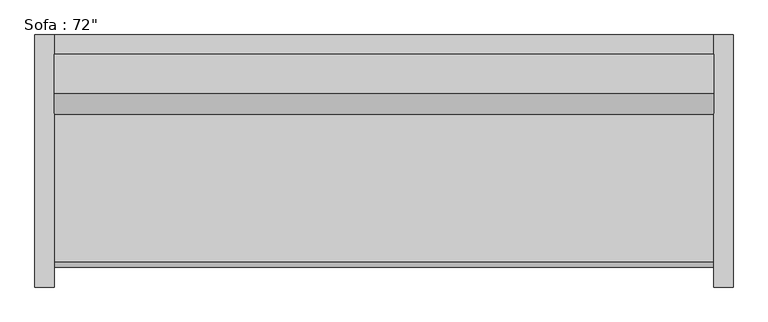
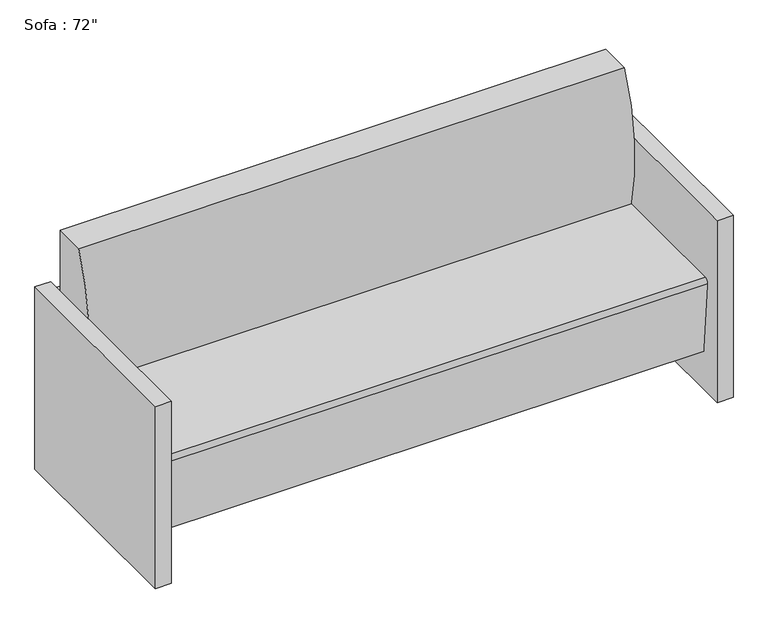
"""IFC4 building model written with IfcOpenShell, lengths in millimetres: furniture geometry."""

from ifc_helpers import new_model, si_unit, point, frame, frame_2d, origin, origin_with_axes, place, context, project, spatial, polyline, circle_curve, trimmed, segment, composite_curve, outline, extrude, source, transform, mapped, element, save


def furniture_a4ffab56(model_context):
    return source(origin(), model_context, "Body", "SweptSolid", [
        extrude(outline(polyline([(-793.2295082, 425.5540984), (-793.2295082, 476.3540984), (933.9704918, 476.3540984), (933.9704918, 425.5540984), (-793.2295082, 425.5540984)])), frame((0.0, 0.0, 457.2), z_axis=(0.0, 0.0, 1.0), x_axis=(1.0, 0.0, 0.0)), (0.0, 0.0, 1.0), 127.0),
        extrude(outline(polyline([(-793.2295082, 425.5540984), (-793.2295082, 476.3540984), (933.9704918, 476.3540984), (933.9704918, 425.5540984), (-793.2295082, 425.5540984)])), frame((0.0, 0.0, 266.7), z_axis=(0.0, 0.0, 1.0), x_axis=(1.0, 0.0, 0.0)), (0.0, 0.0, 1.0), 127.0),
        extrude(outline(polyline([(-793.2295082, 425.5540984), (-793.2295082, 476.3540984), (933.9704918, 476.3540984), (933.9704918, 425.5540984), (-793.2295082, 425.5540984)])), frame((0.0, 0.0, 76.2), z_axis=(0.0, 0.0, 1.0), x_axis=(1.0, 0.0, 0.0)), (0.0, 0.0, 1.0), 127.0),
        extrude(outline(composite_curve([segment(trimmed(circle_curve(frame_2d((926.517198, 542.5300036)), 660.4), [point((286.1764935, 381.0))], [point((323.9540984, 812.8))], False, "CARTESIAN"), True, "CONTINUOUS"), segment(polyline([(323.9540984, 812.8), (425.5540984, 812.8), (425.5540984, 127.9665467), (-111.108343, 127.9665467), (-132.0379563, 367.1931221)]), True, "CONTINUOUS"), segment(trimmed(circle_curve(frame_2d((-119.3862837, 368.3)), 12.7), [point((-132.0379563, 367.1931221))], [point((-119.3862837, 381.0))], False, "CARTESIAN"), True, "CONTINUOUS"), segment(polyline([(-119.3862837, 381.0), (286.1764935, 381.0)]), True, "CONTINUOUS")], self_intersect=False)), frame((-793.2295082, 0.0, 0.0), z_axis=(1.0, 0.0, 0.0), x_axis=(0.0, 1.0, 0.0)), (0.0, 0.0, 1.0), 1727.2),
        extrude(outline(polyline([(-844.0295082, 476.3540984), (-793.2295082, 476.3540984), (-793.2295082, -184.0459016), (-844.0295082, -184.0459016), (-844.0295082, 476.3540984)])), origin_with_axes(), (0.0, 0.0, 1.0), 609.6),
        extrude(outline(polyline([(984.7704918, 476.3540984), (984.7704918, -184.0459016), (933.9704918, -184.0459016), (933.9704918, 476.3540984), (984.7704918, 476.3540984)])), origin_with_axes(), (0.0, 0.0, 1.0), 609.6),
    ])


if __name__ == "__main__":
    model = new_model("IFC4")
    model_context = context("Model", 3, world=origin())
    ifc_project = project(units=[si_unit("LENGTHUNIT", "METRE", prefix="MILLI")], contexts=[model_context])
    site = spatial("IfcSite", under=ifc_project)
    building = spatial("IfcBuilding", under=site)
    placement = place(None, origin())
    furniture_shape = furniture_a4ffab56(model_context)
    element("IfcFurniture", 1, ObjectType="Sofa : 72\"", at=placement, inside=building, context=model_context, shape_type="MappedRepresentation", body=[
        mapped(furniture_shape, transform((0.0, 0.0, 0.0), x_axis=(1.0, 0.0, 0.0), y_axis=(0.0, 1.0, 0.0), z_axis=(0.0, 0.0, 1.0))),
    ])
    save(model, "model.ifc")

# Revit data of these elements
# Type "Sofa : 72\""
#   Assembly Code = "E2020200"
#   Width = 6' - 0"
#   Seat Material = Linen, Beige
#   Frame Material = Cherry
#   Default Elevation = 0
# Element 1 (IfcFurniture, "Sofa : 72\"")
#   Materials on its faces: "Cherry", "Linen, Beige"
# Materials
#   "Linen, Beige": class "Textile", colour RGB 249 239 230, transparency 0, Description = "Linen, beige", Cost = 0
#   "Cherry": class "Wood", colour RGB 226 177 128, transparency 0, Description = "Prunus Serotina", Cost = 0
